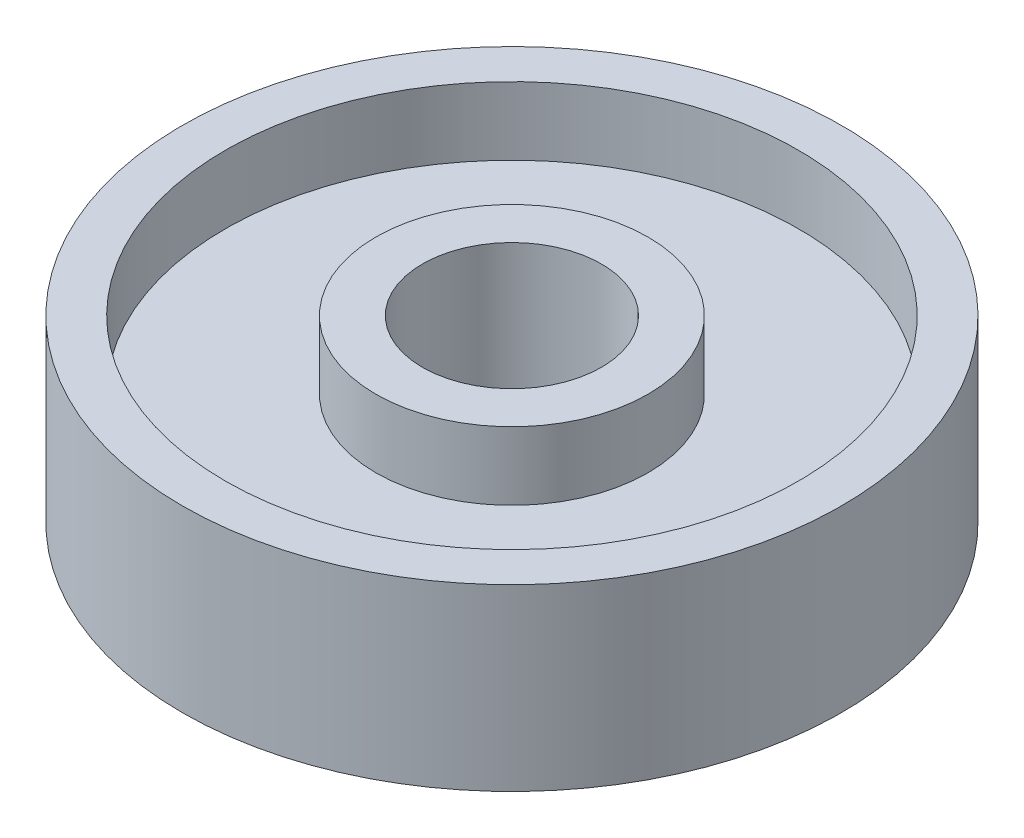
SolidWorks part; units mm, degrees
material "Plain Carbon Steel"
ref_plane "Front Plane" through (0, 0, 0) normal (0, 0, 1) x (1, 0, 0)
ref_plane "Top Plane" through (0, 0, 0) normal (0, 1, 0) x (1, 0, 0)
ref_plane "Right Plane" through (0, 0, 0) normal (1, 0, 0) x (0, 0, -1)
sketch "Base Disc Sketch" plane through (0, 0, 0) normal (0, 1, 0) x (1, 0, 0)
  circle A0 centre (0, 0) radius 46
  dimension "D1" = 92
extrude "Base Disc Ø92" add sketch "Base Disc Sketch" along normal mid plane 6
sketch "Rim Sketch" plane through (0, 3, 0) normal (0, 1, 0) x (1, 0, 0)
  circle A0 centre (0, 0) radius 40
  circle A1 centre (0, 0) radius 46
  dimension "D1" = 92
  dimension "D2" = 80
extrude "Rim Ø92xØ80" add sketch "Rim Sketch" along normal blind 9.5
mirror "Rim Mirror" about plane through (0, 0, 0) normal (0, 1, 0) of "Rim Ø92xØ80"
sketch "Hub Sketch" plane through (0, 12.5, 0) normal (0, 1, 0) x (1, 0, 0)
  circle A0 centre (0, 0) radius 19
  circle A1 centre (0, 0) radius 12.5
  dimension "D1" = 38
  dimension "D2" = 25
extrude "Hub Ø38" add sketch "Hub Sketch" against normal blind 25
sketch "Bore Sketch" plane through (0, 3, 0) normal (0, 1, 0) x (1, 0, 0)
  circle A0 centre (0, 0) radius 12.5
  dimension "D1" = 25
extrude "Bore Ø25" cut sketch "Bore Sketch" against normal blind 25
